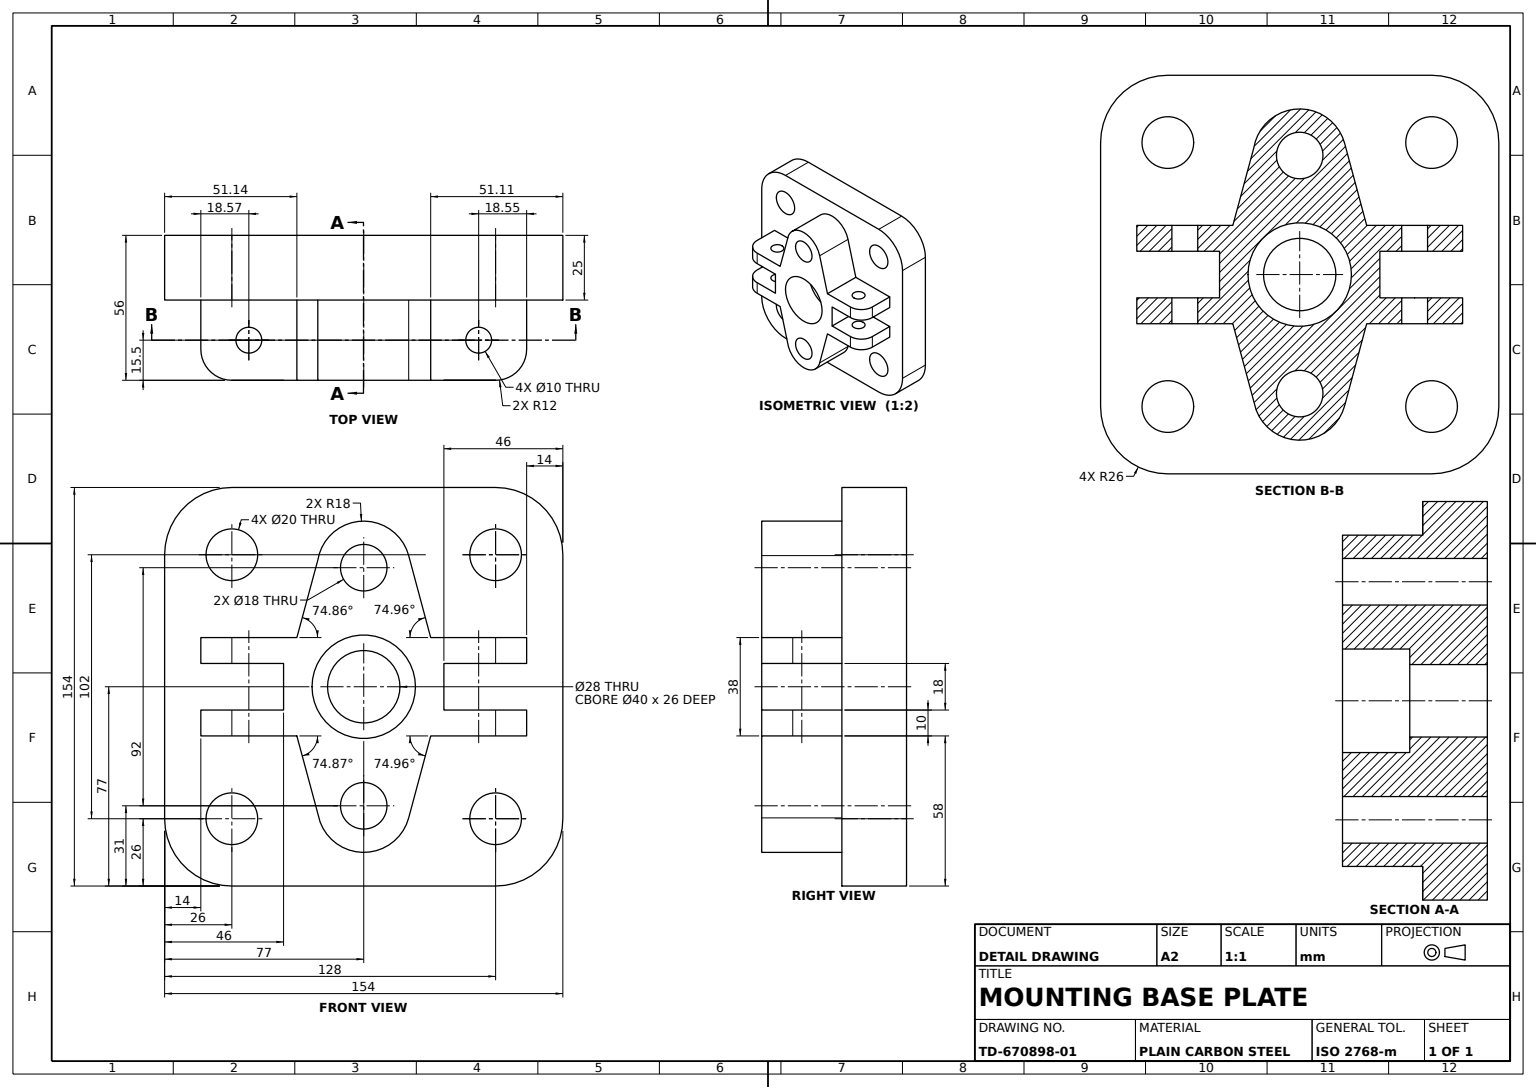
SolidWorks part; units mm, degrees
material "Plain Carbon Steel"
ref_plane "Front Plane" through (0, 0, 0) normal (0, 0, 1) x (1, 0, 0)
ref_plane "Top Plane" through (0, 0, 0) normal (0, 1, 0) x (1, 0, 0)
ref_plane "Right Plane" through (0, 0, 0) normal (1, 0, 0) x (0, 0, -1)
sketch "Base Plate Sketch" plane through (0, 0, 0) normal (0, 0, 1) x (1, 0, 0)
  line L0 (0, 0) -> (154, 0)
  line L1 (154, 0) -> (154, 154)
  line L2 (154, 154) -> (0, 154)
  line L3 (0, 154) -> (0, 0)
  dimension "D1" = 154
  dimension "D2" = 154
extrude "Base Plate" add sketch "Base Plate Sketch" along normal blind 25
fillet "Plate Corner Fillets R26" radius 26 4 edges at (0, 0, 12.5) (154, 0, 12.5) (154, 154, 12.5) (0, 154, 12.5)
sketch "Corner Holes Sketch" plane through (0, 0, 25) normal (0, 0, 1) x (1, 0, 0)
  circle A0 centre (26, 128) radius 10
  circle A1 centre (128, 128) radius 10
  circle A2 centre (128, 26) radius 10
  circle A3 centre (26, 26) radius 10
  dimension "D1" = 20
  dimension "D2" = 20
  dimension "D3" = 20
  dimension "D4" = 20
extrude "Corner Holes 4xØ20" cut sketch "Corner Holes Sketch" against normal blind 25
sketch "Hub Profile Sketch" plane through (0, 0, 25) normal (0, 0, 1) x (1, 0, 0)
  line L0 (77, 77) -> (46, 77) construction
  line L1 (77, 77) -> (108, 77) construction
  line L2 (77, 77) -> (77, 123) construction
  line L3 (77, 77) -> (77, 31) construction
  line L4 (51.1358, 58) -> (60.1329, 24.7151)
  line L5 (51.1425, 96) -> (59.2352, 125.9005)
  line L6 (102.8942, 96) -> (94.3833, 127.6713)
  line L7 (102.8942, 58) -> (94.3833, 26.3287)
  line L8 (46, 86) -> (14, 86)
  line L9 (108, 77) -> (108, 68)
  line L10 (108, 77) -> (108, 86)
  line L11 (46, 77) -> (46, 86)
  line L12 (46, 77) -> (46, 68)
  line L13 (46, 68) -> (14, 68)
  line L14 (14, 68) -> (14, 58)
  line L15 (14, 58) -> (51.1358, 58)
  line L19 (14, 86) -> (14, 96)
  line L20 (14, 96) -> (51.1425, 96)
  line L21 (0, 128) -> (0, 26) construction
  line L22 (108, 86) -> (140, 86)
  line L24 (140, 86) -> (140, 96)
  line L25 (140, 96) -> (102.8942, 96)
  line L26 (108, 68) -> (140, 68)
  line L27 (140, 68) -> (140, 58)
  line L28 (140, 58) -> (102.8942, 58)
  arc A0 (94.3833, 127.6713) -> (59.2352, 125.9005) centre (77, 123) ccw
  arc A1 (59.2635, 27.9314) -> (94.3833, 26.3287) centre (77, 31) ccw
  dimension "D1" = 36
  dimension "D2" = 36
  dimension "D10" = 14
  dimension "D3" = 62
  dimension "D4" = 77
  dimension "D5" = 77
  dimension "D6" = 31
  dimension "D7" = 123
  dimension "D8" = 48.9005
  dimension "D9" = 52.2849
  dimension "D11" = 46
  dimension "D12" = 51.1358
  dimension "D13" = 94.3833
  dimension "D14" = 42
  dimension "D15" = 60
extrude "Central Hub Boss" add sketch "Hub Profile Sketch" along normal blind 31 contours L4 A1 L7 L28 L27 L26 L9 L10 L22 L24 L25 L6 A0 L5 L20 L19 L8 L11 L12 L13 L14 L15
hole_wizard "Centre Tap Drill M20x2.0" positions "Sketch7" profile "Sketch8" hole size "M20x2.0" standard "ISO" end condition through all
sketch "Sketch7" plane through (0, 0, 56) normal (0, 0, 1) x (1, 0, 0)
  point P0 (77, 123)
  point P3 (77, 31)
sketch "Sketch8" plane through (77, 123, 56) normal (1, 0, 0) x (0, -1, 0)
  line L0 (0, 0) -> (0, 56)
  line L1 (0, 56) -> (9, 56)
  line L2 (9, 56) -> (9, 0)
  line L5 (9, 0) -> (0, 0)
  line L11 (0, -6.35) -> (0, 107.95) construction
  dimension "Thru Hole Dia." = 18
  dimension "Thru Hole Depth" = 56
sketch "Counterbore Sketch" plane through (0, 0, 56) normal (0, 0, 1) x (1, 0, 0)
  line L0 (140, 68) -> (140, 58) construction
  line L1 (108, 86) -> (140, 86) construction
  circle A0 centre (77, 77) radius 14
  dimension "D1" = 28
  dimension "D2" = 63
  dimension "D3" = 9
extrude "Counterbore Ø28" cut sketch "Counterbore Sketch" against normal through all
sketch "Bore Step Sketch" plane through (0, 0, 56) normal (0, 0, 1) x (1, 0, 0)
  circle A0 centre (77, 77) radius 20
  dimension "D1" = 40
extrude "Bore Step Cut" cut sketch "Bore Step Sketch" against normal blind 26
sketch "Lug Slot A Sketch" plane through (0, 58, 0) normal (0, -1, 0) x (1, 0, 0)
  line L0 (51.1358, 56) -> (51.1358, 25) construction
  line L1 (14, 25) -> (51.1358, 25) construction
  circle A0 centre (32.5679, 40.5) radius 5
  dimension "D1" = 10
  dimension "D2" = 18.5679
  dimension "D3" = 15.5
extrude "Lug Slot A" cut sketch "Lug Slot A Sketch" against normal through all
sketch "Lug Slot B Sketch" plane through (0, 58, 0) normal (0, -1, 0) x (1, 0, 0)
  line L0 (140, 56) -> (140, 25) construction
  line L1 (140, 25) -> (102.8942, 25) construction
  circle A0 centre (121.4471, 40.5) radius 5
  dimension "D1" = 10
  dimension "D2" = 18.5529
  dimension "D3" = 15.5
extrude "Lug Slot B" cut sketch "Lug Slot B Sketch" against normal through all
fillet "Hub Fillets R12" radius 12 4 edges at (140, 63, 56) (140, 91, 56) (14, 91, 56) (14, 63, 56)
